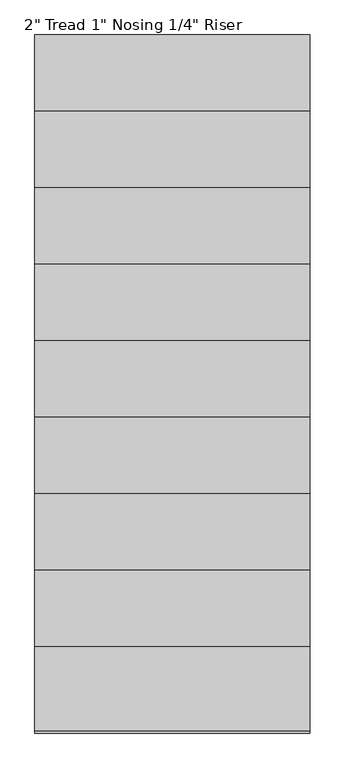
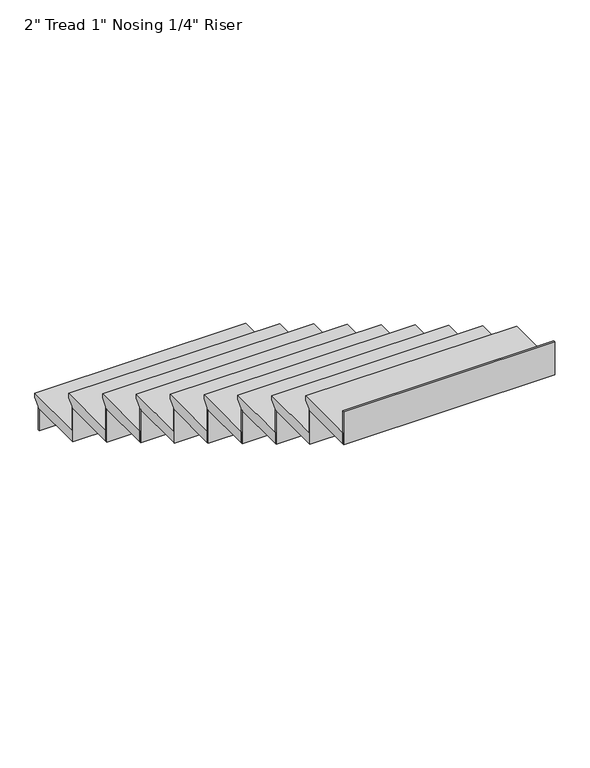
"""IFC4 building model written with IfcOpenShell, lengths in millimetres: stair flight geometry."""

from ifc_helpers import new_model, si_unit, origin, place, context, project, spatial, faceted_brep, source, transform, mapped, element, save


def stair_flight_38cd46e1(model_context):
    return source(origin(), model_context, "Body", "Brep", [
        faceted_brep([(-4315.1137331, -4241.0593836, 133.35), (-4315.1137331, -4241.0593836, 152.4), (-3400.7137331, -4241.0593836, 152.4), (-3400.7137331, -4241.0593836, 133.35), (-4315.1137331, -4266.4593836, 107.95), (-3400.7137331, -4266.4593836, 107.95), (-4315.1137331, -4520.4593836, 152.4), (-3400.7137331, -4520.4593836, 152.4), (-3400.7137331, -4266.4593836, 101.6), (-3400.7137331, -4520.4593836, 101.6), (-4315.1137331, -4520.4593836, 101.6), (-4315.1137331, -4266.4593836, 101.6)], [[[0, 1, 2, 3]], [[4, 0, 3, 5]], [[2, 1, 6, 7]], [[8, 9, 10, 11]], [[2, 7, 9, 8, 5, 3]], [[8, 11, 4, 5]], [[6, 1, 0, 4, 11, 10]], [[7, 6, 10, 9]]]),
        faceted_brep([(-4315.1137331, -4266.4593836, 101.6), (-4315.1137331, -4266.4593836, 0.0), (-4315.1137331, -4272.8093836, 0.0), (-4315.1137331, -4272.8093836, 101.6), (-3400.7137331, -4266.4593836, 101.6), (-3400.7137331, -4272.8093836, 101.6), (-3400.7137331, -4272.8093836, 0.0), (-3400.7137331, -4266.4593836, 0.0)], [[[0, 1, 2, 3]], [[4, 5, 6, 7]], [[1, 0, 4, 7]], [[2, 1, 7, 6]], [[3, 2, 6, 5]], [[0, 3, 5, 4]]]),
        faceted_brep([(-4315.1137331, -4520.4593836, 254.0), (-4315.1137331, -4520.4593836, 101.6), (-4315.1137331, -4526.8093836, 101.6), (-4315.1137331, -4526.8093836, 254.0), (-3400.7137331, -4520.4593836, 254.0), (-3400.7137331, -4526.8093836, 254.0), (-3400.7137331, -4526.8093836, 101.6), (-3400.7137331, -4520.4593836, 101.6)], [[[0, 1, 2, 3]], [[4, 5, 6, 7]], [[1, 0, 4, 7]], [[2, 1, 7, 6]], [[3, 2, 6, 5]], [[0, 3, 5, 4]]]),
        faceted_brep([(-3400.7137331, -4495.0593836, 304.8), (-4315.1137331, -4495.0593836, 304.8), (-4315.1137331, -4774.4593836, 304.8), (-3400.7137331, -4774.4593836, 304.8), (-3400.7137331, -4520.4593836, 254.0), (-3400.7137331, -4774.4593836, 254.0), (-4315.1137331, -4774.4593836, 254.0), (-4315.1137331, -4520.4593836, 254.0), (-3400.7137331, -4520.4593836, 260.35), (-3400.7137331, -4495.0593836, 285.75), (-4315.1137331, -4520.4593836, 260.35), (-4315.1137331, -4495.0593836, 285.75)], [[[0, 1, 2, 3]], [[4, 5, 6, 7]], [[0, 3, 5, 4, 8, 9]], [[4, 7, 10, 8]], [[2, 1, 11, 10, 7, 6]], [[3, 2, 6, 5]], [[11, 1, 0, 9]], [[10, 11, 9, 8]]]),
        faceted_brep([(-4315.1137331, -4774.4593836, 406.4), (-4315.1137331, -4774.4593836, 254.0), (-4315.1137331, -4780.8093836, 254.0), (-4315.1137331, -4780.8093836, 406.4), (-3400.7137331, -4774.4593836, 406.4), (-3400.7137331, -4780.8093836, 406.4), (-3400.7137331, -4780.8093836, 254.0), (-3400.7137331, -4774.4593836, 254.0)], [[[0, 1, 2, 3]], [[4, 5, 6, 7]], [[1, 0, 4, 7]], [[2, 1, 7, 6]], [[3, 2, 6, 5]], [[0, 3, 5, 4]]]),
        faceted_brep([(-3400.7137331, -4749.0593836, 457.2), (-4315.1137331, -4749.0593836, 457.2), (-4315.1137331, -5028.4593836, 457.2), (-3400.7137331, -5028.4593836, 457.2), (-3400.7137331, -4774.4593836, 406.4), (-3400.7137331, -5028.4593836, 406.4), (-4315.1137331, -5028.4593836, 406.4), (-4315.1137331, -4774.4593836, 406.4), (-3400.7137331, -4774.4593836, 412.75), (-3400.7137331, -4749.0593836, 438.15), (-4315.1137331, -4774.4593836, 412.75), (-4315.1137331, -4749.0593836, 438.15)], [[[0, 1, 2, 3]], [[4, 5, 6, 7]], [[0, 3, 5, 4, 8, 9]], [[4, 7, 10, 8]], [[2, 1, 11, 10, 7, 6]], [[3, 2, 6, 5]], [[11, 1, 0, 9]], [[10, 11, 9, 8]]]),
        faceted_brep([(-4315.1137331, -5028.4593836, 558.8), (-4315.1137331, -5028.4593836, 406.4), (-4315.1137331, -5034.8093836, 406.4), (-4315.1137331, -5034.8093836, 558.8), (-3400.7137331, -5028.4593836, 558.8), (-3400.7137331, -5034.8093836, 558.8), (-3400.7137331, -5034.8093836, 406.4), (-3400.7137331, -5028.4593836, 406.4)], [[[0, 1, 2, 3]], [[4, 5, 6, 7]], [[1, 0, 4, 7]], [[2, 1, 7, 6]], [[3, 2, 6, 5]], [[0, 3, 5, 4]]]),
        faceted_brep([(-3400.7137331, -5003.0593836, 609.6), (-4315.1137331, -5003.0593836, 609.6), (-4315.1137331, -5282.4593836, 609.6), (-3400.7137331, -5282.4593836, 609.6), (-3400.7137331, -5028.4593836, 558.8), (-3400.7137331, -5282.4593836, 558.8), (-4315.1137331, -5282.4593836, 558.8), (-4315.1137331, -5028.4593836, 558.8), (-3400.7137331, -5028.4593836, 565.15), (-3400.7137331, -5003.0593836, 590.55), (-4315.1137331, -5028.4593836, 565.15), (-4315.1137331, -5003.0593836, 590.55)], [[[0, 1, 2, 3]], [[4, 5, 6, 7]], [[0, 3, 5, 4, 8, 9]], [[4, 7, 10, 8]], [[2, 1, 11, 10, 7, 6]], [[3, 2, 6, 5]], [[11, 1, 0, 9]], [[10, 11, 9, 8]]]),
        faceted_brep([(-4315.1137331, -5282.4593836, 711.2), (-4315.1137331, -5282.4593836, 558.8), (-4315.1137331, -5288.8093836, 558.8), (-4315.1137331, -5288.8093836, 711.2), (-3400.7137331, -5282.4593836, 711.2), (-3400.7137331, -5288.8093836, 711.2), (-3400.7137331, -5288.8093836, 558.8), (-3400.7137331, -5282.4593836, 558.8)], [[[0, 1, 2, 3]], [[4, 5, 6, 7]], [[1, 0, 4, 7]], [[2, 1, 7, 6]], [[3, 2, 6, 5]], [[0, 3, 5, 4]]]),
        faceted_brep([(-3400.7137331, -5257.0593836, 762.0), (-4315.1137331, -5257.0593836, 762.0), (-4315.1137331, -5536.4593836, 762.0), (-3400.7137331, -5536.4593836, 762.0), (-3400.7137331, -5282.4593836, 711.2), (-3400.7137331, -5536.4593836, 711.2), (-4315.1137331, -5536.4593836, 711.2), (-4315.1137331, -5282.4593836, 711.2), (-3400.7137331, -5282.4593836, 717.55), (-3400.7137331, -5257.0593836, 742.95), (-4315.1137331, -5282.4593836, 717.55), (-4315.1137331, -5257.0593836, 742.95)], [[[0, 1, 2, 3]], [[4, 5, 6, 7]], [[0, 3, 5, 4, 8, 9]], [[4, 7, 10, 8]], [[2, 1, 11, 10, 7, 6]], [[3, 2, 6, 5]], [[11, 1, 0, 9]], [[10, 11, 9, 8]]]),
        faceted_brep([(-4315.1137331, -5536.4593836, 863.6), (-4315.1137331, -5536.4593836, 711.2), (-4315.1137331, -5542.8093836, 711.2), (-4315.1137331, -5542.8093836, 863.6), (-3400.7137331, -5536.4593836, 863.6), (-3400.7137331, -5542.8093836, 863.6), (-3400.7137331, -5542.8093836, 711.2), (-3400.7137331, -5536.4593836, 711.2)], [[[0, 1, 2, 3]], [[4, 5, 6, 7]], [[1, 0, 4, 7]], [[2, 1, 7, 6]], [[3, 2, 6, 5]], [[0, 3, 5, 4]]]),
        faceted_brep([(-3400.7137331, -5511.0593836, 914.4), (-4315.1137331, -5511.0593836, 914.4), (-4315.1137331, -5790.4593836, 914.4), (-3400.7137331, -5790.4593836, 914.4), (-3400.7137331, -5536.4593836, 863.6), (-3400.7137331, -5790.4593836, 863.6), (-4315.1137331, -5790.4593836, 863.6), (-4315.1137331, -5536.4593836, 863.6), (-3400.7137331, -5536.4593836, 869.95), (-3400.7137331, -5511.0593836, 895.35), (-4315.1137331, -5536.4593836, 869.95), (-4315.1137331, -5511.0593836, 895.35)], [[[0, 1, 2, 3]], [[4, 5, 6, 7]], [[0, 3, 5, 4, 8, 9]], [[4, 7, 10, 8]], [[2, 1, 11, 10, 7, 6]], [[3, 2, 6, 5]], [[11, 1, 0, 9]], [[10, 11, 9, 8]]]),
        faceted_brep([(-4315.1137331, -5790.4593836, 1016.0), (-4315.1137331, -5790.4593836, 863.6), (-4315.1137331, -5796.8093836, 863.6), (-4315.1137331, -5796.8093836, 1016.0), (-3400.7137331, -5790.4593836, 1016.0), (-3400.7137331, -5796.8093836, 1016.0), (-3400.7137331, -5796.8093836, 863.6), (-3400.7137331, -5790.4593836, 863.6)], [[[0, 1, 2, 3]], [[4, 5, 6, 7]], [[1, 0, 4, 7]], [[2, 1, 7, 6]], [[3, 2, 6, 5]], [[0, 3, 5, 4]]]),
        faceted_brep([(-3400.7137331, -5765.0593836, 1066.8), (-4315.1137331, -5765.0593836, 1066.8), (-4315.1137331, -6044.4593836, 1066.8), (-3400.7137331, -6044.4593836, 1066.8), (-3400.7137331, -5790.4593836, 1016.0), (-3400.7137331, -6044.4593836, 1016.0), (-4315.1137331, -6044.4593836, 1016.0), (-4315.1137331, -5790.4593836, 1016.0), (-3400.7137331, -5790.4593836, 1022.35), (-3400.7137331, -5765.0593836, 1047.75), (-4315.1137331, -5790.4593836, 1022.35), (-4315.1137331, -5765.0593836, 1047.75)], [[[0, 1, 2, 3]], [[4, 5, 6, 7]], [[0, 3, 5, 4, 8, 9]], [[4, 7, 10, 8]], [[2, 1, 11, 10, 7, 6]], [[3, 2, 6, 5]], [[11, 1, 0, 9]], [[10, 11, 9, 8]]]),
        faceted_brep([(-4315.1137331, -6044.4593836, 1168.4), (-4315.1137331, -6044.4593836, 1016.0), (-4315.1137331, -6050.8093836, 1016.0), (-4315.1137331, -6050.8093836, 1168.4), (-3400.7137331, -6044.4593836, 1168.4), (-3400.7137331, -6050.8093836, 1168.4), (-3400.7137331, -6050.8093836, 1016.0), (-3400.7137331, -6044.4593836, 1016.0)], [[[0, 1, 2, 3]], [[4, 5, 6, 7]], [[1, 0, 4, 7]], [[2, 1, 7, 6]], [[3, 2, 6, 5]], [[0, 3, 5, 4]]]),
        faceted_brep([(-3400.7137331, -6019.0593836, 1219.2), (-4315.1137331, -6019.0593836, 1219.2), (-4315.1137331, -6298.4593836, 1219.2), (-3400.7137331, -6298.4593836, 1219.2), (-3400.7137331, -6044.4593836, 1168.4), (-3400.7137331, -6298.4593836, 1168.4), (-4315.1137331, -6298.4593836, 1168.4), (-4315.1137331, -6044.4593836, 1168.4), (-3400.7137331, -6044.4593836, 1174.75), (-3400.7137331, -6019.0593836, 1200.15), (-4315.1137331, -6044.4593836, 1174.75), (-4315.1137331, -6019.0593836, 1200.15)], [[[0, 1, 2, 3]], [[4, 5, 6, 7]], [[0, 3, 5, 4, 8, 9]], [[4, 7, 10, 8]], [[2, 1, 11, 10, 7, 6]], [[3, 2, 6, 5]], [[11, 1, 0, 9]], [[10, 11, 9, 8]]]),
        faceted_brep([(-4315.1137331, -6552.4593836, 1473.2), (-4315.1137331, -6552.4593836, 1320.8), (-4315.1137331, -6558.8093836, 1320.8), (-4315.1137331, -6558.8093836, 1473.2), (-3400.7137331, -6552.4593836, 1473.2), (-3400.7137331, -6558.8093836, 1473.2), (-3400.7137331, -6558.8093836, 1320.8), (-3400.7137331, -6552.4593836, 1320.8)], [[[0, 1, 2, 3]], [[4, 5, 6, 7]], [[1, 0, 4, 7]], [[2, 1, 7, 6]], [[3, 2, 6, 5]], [[0, 3, 5, 4]]]),
        faceted_brep([(-4315.1137331, -6298.4593836, 1320.8), (-4315.1137331, -6298.4593836, 1168.4), (-4315.1137331, -6304.8093836, 1168.4), (-4315.1137331, -6304.8093836, 1320.8), (-3400.7137331, -6298.4593836, 1320.8), (-3400.7137331, -6304.8093836, 1320.8), (-3400.7137331, -6304.8093836, 1168.4), (-3400.7137331, -6298.4593836, 1168.4)], [[[0, 1, 2, 3]], [[4, 5, 6, 7]], [[1, 0, 4, 7]], [[2, 1, 7, 6]], [[3, 2, 6, 5]], [[0, 3, 5, 4]]]),
        faceted_brep([(-3400.7137331, -6552.4593836, 1371.6), (-3400.7137331, -6527.0593836, 1371.6), (-3400.7137331, -6273.0593836, 1371.6), (-4315.1137331, -6273.0593836, 1371.6), (-4315.1137331, -6552.4593836, 1371.6), (-3400.7137331, -6527.0593836, 1320.8), (-3400.7137331, -6552.4593836, 1320.8), (-4315.1137331, -6552.4593836, 1320.8), (-4315.1137331, -6298.4593836, 1320.8), (-3400.7137331, -6298.4593836, 1320.8), (-3400.7137331, -6298.4593836, 1327.15), (-3400.7137331, -6273.0593836, 1352.55), (-4315.1137331, -6298.4593836, 1327.15), (-4315.1137331, -6273.0593836, 1352.55)], [[[0, 1, 2, 3, 4]], [[5, 6, 7, 8, 9]], [[1, 0, 6, 5]], [[2, 1, 5, 9, 10, 11]], [[9, 8, 12, 10]], [[4, 3, 13, 12, 8, 7]], [[0, 4, 7, 6]], [[13, 3, 2, 11]], [[12, 13, 11, 10]]]),
    ])


if __name__ == "__main__":
    model = new_model("IFC4")
    model_context = context("Model", 3, world=origin())
    ifc_project = project(units=[si_unit("LENGTHUNIT", "METRE", prefix="MILLI")], contexts=[model_context])
    site = spatial("IfcSite", under=ifc_project)
    building = spatial("IfcBuilding", under=site)
    placement = place(None, origin())
    stair_flight_shape = stair_flight_38cd46e1(model_context)
    element("IfcStairFlight", 1, ObjectType="2\" Tread 1\" Nosing 1/4\" Riser", at=placement, inside=building, context=model_context, shape_type="MappedRepresentation", body=[
        mapped(stair_flight_shape, transform((0.0, 0.0, 0.0), x_axis=(1.0, 0.0, 0.0), y_axis=(0.0, 1.0, 0.0), z_axis=(0.0, 0.0, 1.0))),
    ])
    save(model, "model.ifc")
